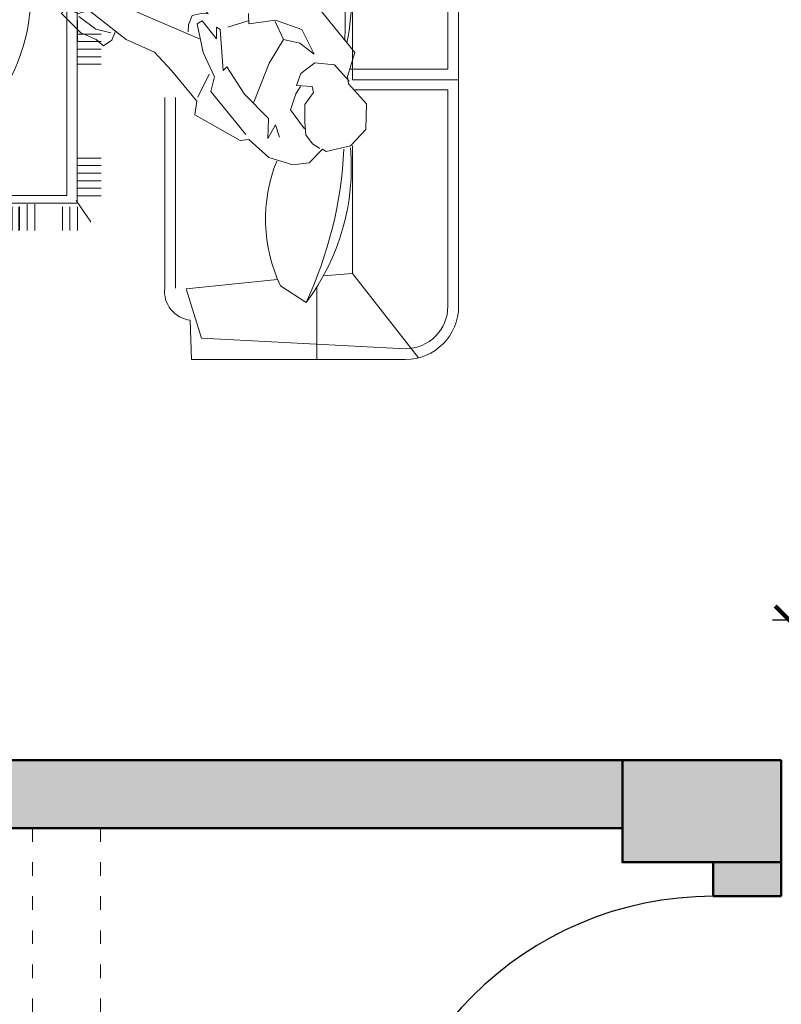
# Model space of a CAD drawing. Units: inches. Extents: x 375 to 1122, y 27 to 1069.
# Tile 5 of 155: x 599 to 667, y 313 to 400. Entities that reach past the tile are written whole.
import ezdxf

# ---------------------------------------------------------------- set-up
doc = ezdxf.new("R2010")
doc.units = ezdxf.units.IN
doc.linetypes.add('ACAD_ISO03W100', pattern=[30, 12, -18])
for name, color, linetype, lineweight in [('A-ANNO-DIMS', 2, 'Continuous', 18), ('A-COLS-PATT', 10, 'Continuous', 13), ('A-WALL-OVHD', 77, 'ACAD_ISO03W100', 18), ('A-WALL-PATT', 252, 'Continuous', 13), ('Columns', 10, 'Continuous', 50), ('Doors', 150, 'Continuous', 25), ('Furniture', 30, 'Continuous', 18), ('Walls', 250, 'Continuous', 50)]:
    doc.layers.add(name, color=color, linetype=linetype, lineweight=lineweight)
doc.styles.get("Standard").update_dxf_attribs({"font": 'arial.ttf'})
doc.dimstyles.new('ISO-25', dxfattribs={"dimtxt": 12, "dimasz": 2.5, "dimexe": 1.5, "dimexo": 1.5, "dimtad": 1, "dimdec": 1, "dimlunit": 3, "dimtxsty": 'Standard', "dimblk": 'ARCHTICK', "dimcen": 2.5, "dimadec": 0, "dimazin": 0, "dimtfac": 1, "dimtdec": 1, "dimtmove": 0, "dimatfit": 3, "dimfxl": 1.5, "dimfxlon": 1, "dimarcsym": 0})

# ---------------------------------------------------------------- blocks, each defined once
blk = doc.blocks.new('*U10')
for p, q in [((-30, 0), (-30, 4)), ((0, 0), (0, 4))]:
    blk.add_line(p, q)
blk.add_lwpolyline([(0, 0), (0, -30), (-1.75, -30), (-1.75, 0)], close=True)
blk.add_arc((0, 0), 30, 180, 270)
blk = doc.blocks.new('A$C4DC51D13')
for p, q in [((3265.3, 2996.2), (1188.4, 2996.2)), ((1895.2, 2134), (1895.2, 2996.2)), ((2559.6, 2996.2), (2559.6, 2617.8)), ((1188.4, 2962.7), (1862.1, 2962.7)), ((1862.1, 2134), (1862.1, 2962.7)), ((1928.3, 2961.6), (2524.2, 2961.6)), ((1928.3, 2134), (1928.3, 2961.6)), ((2524.2, 2961.6), (2524.2, 2658.6)), ((2590.4, 2962.7), (2590.4, 2654.5)), ((3265.3, 2962.7), (2590.4, 2962.7)), ((277.4, 2939.6), (277.4, 2141.8)), ((943, 2103.5), (943, 2936.7)), ((1018.2, 2892.3), (232.2, 2892.3)), ((3778.5, 2897), (3631.2, 2747.3)), ((4008.9, 2375.5), (3778.5, 2897)), ((4156.2, 2525.2), (3778.5, 2897)), ((304, 2865.7), (304, 2253.3)), ((916.4, 2865.7), (304, 2865.7)), ((916.4, 2253.3), (916.4, 2865.7)), ((1290.4, 2664.8), (1028, 2870.9)), ((3163.3, 2664.8), (3425.7, 2870.9)), ((1022.9, 2163.8), (1022.9, 2830.3)), ((1056, 2830.3), (1081, 2194.8)), ((3397.7, 2830.3), (3364.5, 2194.8)), ((3430.8, 2163.8), (3430.8, 2830.3)), ((4008.9, 2375.5), (3631.2, 2747.3)), ((423.7, 2370.8), (776.6, 2723.7)), ((427.4, 2727.4), (772.8, 2367.1)), ((502.2, 2648.3), (502.2, 2701.8)), ((506.4, 2652.2), (506.4, 2704.4)), ((510.6, 2655.8), (510.6, 2706.9)), ((514.9, 2659.2), (514.9, 2709.2)), ((519.1, 2662.3), (519.1, 2711.3)), ((523.3, 2665.1), (523.3, 2713.4)), ((527.5, 2667.8), (527.5, 2715.2)), ((531.8, 2670.2), (531.8, 2717)), ((536, 2672.5), (536, 2718.7)), ((540.2, 2674.6), (540.2, 2720.2)), ((544.4, 2676.5), (544.4, 2721.6)), ((548.7, 2678.2), (548.7, 2722.9)), ((650.1, 2678.8), (650.1, 2723.3)), ((654.3, 2677.1), (654.3, 2722)), ((658.6, 2675.2), (658.6, 2720.7)), ((662.8, 2673.2), (662.8, 2719.2)), ((667, 2671), (667, 2717.6)), ((668.5, 2670.2), (668.5, 2717)), ((671.2, 2668.6), (671.2, 2715.9)), ((672.7, 2667.8), (672.7, 2715.2)), ((675.5, 2666.1), (675.5, 2714)), ((676.9, 2665.1), (676.9, 2713.4)), ((679.7, 2663.3), (679.7, 2712)), ((681.1, 2662.3), (681.1, 2711.3)), ((683.9, 2660.3), (683.9, 2709.9)), ((685.4, 2659.2), (685.4, 2709.2)), ((688.1, 2657), (688.1, 2707.7)), ((689.6, 2655.8), (689.6, 2706.9)), ((692.4, 2653.5), (692.4, 2705.3)), ((693.8, 2652.2), (693.8, 2704.4)), ((696.6, 2649.6), (696.6, 2702.7)), ((698, 2648.3), (698, 2701.8)), ((465.8, 2671.5), (534.1, 2671.5)), ((468.4, 2596.6), (468.4, 2674.3)), ((469.8, 2675.7), (542.8, 2675.7)), ((472.6, 2606.7), (472.6, 2678.5)), ((476.8, 2615), (476.8, 2682.5)), ((481, 2622.2), (481, 2686.2)), ((485.3, 2628.5), (485.3, 2689.7)), ((489.5, 2634.2), (489.5, 2693)), ((493.7, 2639.3), (493.7, 2696.1)), ((497.9, 2644), (497.9, 2699.1)), ((657.4, 2675.7), (730.4, 2675.7)), ((734.5, 2671.5), (666.1, 2671.5)), ((666.1, 2671.5), (734.5, 2671.5)), ((700.8, 2645.5), (700.8, 2700)), ((702.3, 2644), (702.3, 2699.1)), ((705, 2641), (705, 2697.2)), ((706.5, 2639.3), (706.5, 2696.1)), ((709.3, 2636), (709.3, 2694.1)), ((710.7, 2634.2), (710.7, 2693)), ((713.5, 2630.5), (713.5, 2690.9)), ((714.9, 2628.5), (714.9, 2689.7)), ((717.7, 2624.4), (717.7, 2687.4)), ((719.2, 2622.2), (719.2, 2686.2)), ((722, 2617.6), (722, 2683.8)), ((723.4, 2615), (723.4, 2682.5)), ((726.2, 2609.7), (726.2, 2679.9)), ((727.6, 2606.7), (727.6, 2678.5)), ((730.4, 2600.3), (730.4, 2675.7)), ((731.9, 2596.6), (731.9, 2674.3)), ((734.6, 2588.4), (734.6, 2671.3)), ((3631.7, 2676.6), (3938.2, 2375)), ((443, 2453.4), (443, 2641.1)), ((443.5, 2641.9), (496, 2641.9)), ((446.1, 2646.1), (500, 2646.1)), ((447.2, 2446.7), (447.2, 2647.8)), ((448.9, 2650.4), (504.4, 2650.4)), ((451.5, 2440.6), (451.5, 2654)), ((451.9, 2654.6), (509.2, 2654.6)), ((455.1, 2658.8), (514.4, 2658.8)), ((455.7, 2434.9), (455.7, 2659.6)), ((458.4, 2663.1), (520.2, 2663.1)), ((459.9, 2558.8), (459.9, 2664.9)), ((462, 2667.3), (526.7, 2667.3)), ((464.1, 2583.3), (464.1, 2669.7)), ((489.5, 2667.3), (489.5, 2633.5)), ((738.2, 2667.3), (673.5, 2667.3)), ((673.5, 2667.3), (738.2, 2667.3)), ((741.8, 2663.1), (680, 2663.1)), ((680, 2663.1), (741.8, 2663.1)), ((745.2, 2658.8), (685.8, 2658.8)), ((685.8, 2658.8), (745.2, 2658.8)), ((748.3, 2654.6), (691, 2654.6)), ((691, 2654.6), (748.3, 2654.6)), ((751.3, 2650.4), (695.8, 2650.4)), ((695.8, 2650.4), (751.3, 2650.4)), ((754.1, 2646.1), (700.2, 2646.1)), ((700.2, 2646.1), (754.1, 2646.1)), ((756.7, 2641.9), (704.2, 2641.9)), ((704.2, 2641.9), (756.7, 2641.9)), ((736.1, 2583.3), (736.1, 2669.7)), ((738.9, 2570.4), (738.9, 2666.6)), ((740.3, 2558.8), (740.3, 2664.9)), ((743.1, 2433.1), (743.1, 2661.5)), ((744.5, 2434.9), (744.5, 2659.6)), ((747.3, 2438.6), (747.3, 2656)), ((748.8, 2440.6), (748.8, 2654)), ((751.5, 2444.5), (751.5, 2650)), ((753, 2446.7), (753, 2647.8)), ((755.8, 2451.1), (755.8, 2643.5)), ((757.2, 2453.4), (757.2, 2641.1)), ((1283.3, 2574.2), (1290.4, 2664.8)), ((1290.4, 2664.8), (1894.7, 2664.8)), ((1895.2, 2663.7), (2557.3, 2663.7)), ((2603.6, 2664.8), (2559, 2664.8)), ((3163.3, 2664.8), (2764.7, 2664.8)), ((3170.4, 2574.2), (3163.3, 2664.8)), ((429.1, 2612.3), (475.4, 2612.3)), ((430.3, 2479), (430.3, 2615.5)), ((430.7, 2616.6), (477.7, 2616.6)), ((432.5, 2620.8), (480.2, 2620.8)), ((434.5, 2469.3), (434.5, 2625.2)), ((434.5, 2625), (482.9, 2625)), ((436.5, 2629.2), (485.8, 2629.2)), ((438.7, 2633.5), (488.9, 2633.5)), ((438.8, 2460.9), (438.8, 2633.6)), ((441, 2637.7), (492.3, 2637.7)), ((759.2, 2637.7), (707.9, 2637.7)), ((707.9, 2637.7), (759.2, 2637.7)), ((761.5, 2633.5), (711.3, 2633.5)), ((711.3, 2633.5), (761.5, 2633.5)), ((763.7, 2629.2), (714.4, 2629.2)), ((714.4, 2629.2), (763.7, 2629.2)), ((765.8, 2625), (717.3, 2625)), ((767.7, 2620.8), (720, 2620.8)), ((769.5, 2616.6), (722.5, 2616.6)), ((771.1, 2612.3), (724.8, 2612.3)), ((760, 2458.3), (760, 2636.3)), ((761.4, 2460.9), (761.4, 2633.6)), ((764.2, 2466.3), (764.2, 2628.2)), ((765.7, 2469.3), (765.7, 2625.2)), ((1798, 2530.2), (1812.1, 2637.9)), ((419.8, 2578.5), (462.9, 2578.5)), ((420.6, 2582.7), (464, 2582.7)), ((421.5, 2587), (465.2, 2587)), ((422.5, 2591.2), (466.5, 2591.2)), ((423.6, 2595.4), (467.9, 2595.4)), ((424.8, 2599.7), (469.6, 2599.7)), ((426.1, 2603.9), (471.3, 2603.9)), ((426.1, 2490.7), (426.1, 2603.9)), ((427.5, 2608.1), (473.3, 2608.1)), ((772.7, 2608.1), (726.9, 2608.1)), ((774.1, 2603.9), (728.9, 2603.9)), ((775.4, 2599.7), (730.7, 2599.7)), ((776.6, 2595.4), (732.3, 2595.4)), ((777.7, 2591.2), (733.7, 2591.2)), ((778.7, 2587), (735.1, 2587)), ((779.6, 2582.7), (736.2, 2582.7)), ((780.4, 2578.5), (737.3, 2578.5)), ((1895.5, 2582.2), (1932.3, 2494.6)), ((417.1, 2548.9), (459.4, 2548.9)), ((417.2, 2553.2), (459.6, 2553.2)), ((417.4, 2557.4), (459.8, 2557.4)), ((417.7, 2561.6), (460.2, 2561.6)), ((418.1, 2565.8), (460.7, 2565.8)), ((418.5, 2570.1), (461.3, 2570.1)), ((419.1, 2574.3), (462.1, 2574.3)), ((781.1, 2574.3), (738.2, 2574.3)), ((781.7, 2570.1), (738.9, 2570.1)), ((782.2, 2565.8), (739.6, 2565.8)), ((782.5, 2561.6), (740.1, 2561.6)), ((782.8, 2557.4), (740.4, 2557.4)), ((783, 2553.2), (740.7, 2553.2)), ((783.1, 2548.9), (740.8, 2548.9)), ((1022.9, 2554.4), (1249.6, 2554.4)), ((3430.8, 2554.4), (3204.1, 2554.4)), ((417.1, 2544.7), (459.5, 2544.7)), ((417.2, 2540.5), (459.6, 2540.5)), ((417.5, 2536.3), (459.9, 2536.3)), ((417.8, 2532), (460.3, 2532)), ((418.2, 2527.8), (460.8, 2527.8)), ((418.7, 2523.6), (461.4, 2523.6)), ((419.3, 2519.4), (462.2, 2519.4)), ((459.9, 2429.7), (459.9, 2535.7)), ((781, 2519.4), (738, 2519.4)), ((781.6, 2523.6), (738.8, 2523.6)), ((782.1, 2527.8), (739.4, 2527.8)), ((782.5, 2532), (740, 2532)), ((740.3, 2429.7), (740.3, 2535.7)), ((782.8, 2536.3), (740.4, 2536.3)), ((783, 2540.5), (740.6, 2540.5)), ((783.1, 2544.7), (740.8, 2544.7)), ((1200, 2520.5), (1251.9, 2440.8)), ((2559, 2535.8), (2557.3, 2535.8)), ((3253.7, 2520.5), (3201.8, 2440.8)), ((4008.9, 2375.5), (4156.2, 2525.2)), ((1243.2, 2146.7), (1272.2, 2431.8)), ((3210.5, 2146.7), (3181.5, 2431.8)), ((304, 2253.3), (916.4, 2253.3)), ((242.9, 2226.7), (1018.2, 2226.7)), ((1081, 2194.8), (1243.2, 2146.7)), ((3364.5, 2194.8), (3210.5, 2146.7)), ((1145.1, 2159.3), (1022.9, 2163.8)), ((1145.1, 2159.3), (1243.2, 2146.7)), ((2590.4, 2164.3), (2590.4, 2134)), ((3308.6, 2159.3), (3210.5, 2146.7)), ((3308.6, 2159.3), (3430.8, 2163.8)), ((498.8, 1837.1), (382.1, 2139.5)), ((1040.3, 1942.9), (421.2, 2132.6)), ((1244.8, 2113), (1243.2, 2146.7)), ((3208.9, 2113), (3210.5, 2146.7)), ((411.8, 2101.9), (992.6, 1890.2)), ((1839.5, 2113), (1244.8, 2113)), ((2308.5, 2111.9), (1950.4, 2111.9)), ((2614.2, 2113), (3208.9, 2113)), ((1839.5, 2079.9), (1244.8, 2079.9)), ((2322.1, 2078.8), (1950.4, 2078.8)), ((2614.2, 2079.9), (3208.9, 2079.9)), ((220.3, 2026), (19.3, 1370.1)), ((677.4, 2054.1), (612.9, 1843.6)), ((251.1, 2016.6), (37.1, 1314.7)), ((1009.7, 1828.1), (1040.3, 1942.9)), ((658.5, 1880), (717.8, 1809.1)), ((992.6, 1890.2), (993.4, 1733.4)), ((1158.3, 1784.3), (1158.3, 1858.2)), ((1181.8, 1784.3), (1181.8, 1858.2)), ((1205.3, 1784.3), (1205.3, 1858.2)), ((1228.8, 1784.3), (1228.8, 1858.2)), ((1252.2, 1784.3), (1252.2, 1858.2)), ((1319.4, 1784.3), (1319.4, 1858.2)), ((1342.9, 1784.3), (1342.9, 1858.2)), ((1366.3, 1784.3), (1366.3, 1858.2)), ((1389.8, 1784.3), (1389.8, 1858.2)), ((1413.3, 1784.3), (1413.3, 1858.2)), ((1436.8, 1784.3), (1436.8, 1858.2)), ((1460.2, 1784.3), (1460.2, 1858.2)), ((1483.7, 1784.3), (1483.7, 1858.2)), ((1507.2, 1784.3), (1507.2, 1858.2)), ((1530.7, 1784.3), (1530.7, 1858.2)), ((1554.1, 1784.3), (1554.1, 1858.2)), ((1577.6, 1784.3), (1577.6, 1858.2)), ((1714.2, 1784.3), (1714.2, 1858.2)), ((1737.6, 1784.3), (1737.6, 1858.2)), ((1761.1, 1784.3), (1761.1, 1858.2)), ((1784.6, 1784.3), (1784.6, 1858.2)), ((1808.1, 1784.3), (1808.1, 1858.2)), ((1831.5, 1784.3), (1831.5, 1858.2)), ((1855, 1784.3), (1855, 1858.2)), ((1878.5, 1784.3), (1878.5, 1858.2)), ((1902, 1784.3), (1902, 1858.2)), ((2050.7, 1784.3), (2050.7, 1858.2)), ((2074.2, 1784.3), (2074.2, 1858.2)), ((2097.7, 1784.3), (2097.7, 1858.2)), ((2121.1, 1784.3), (2121.1, 1858.2)), ((2144.6, 1784.3), (2144.6, 1858.2)), ((2168.1, 1784.3), (2168.1, 1858.2)), ((2191.6, 1782.4), (2191.6, 1856.3)), ((2238.5, 1785.1), (2238.5, 1859)), ((2262, 1784.3), (2262, 1858.2)), ((2285.4, 1784.3), (2285.4, 1858.2)), ((2543.7, 1784.3), (2543.7, 1858.2)), ((2567.1, 1784.3), (2567.1, 1858.2)), ((2590.6, 1784.3), (2590.6, 1858.2)), ((2614.1, 1784.3), (2614.1, 1858.2)), ((2661, 1784.3), (2661, 1858.2)), ((2684.5, 1784.3), (2684.5, 1858.2)), ((2708, 1772.3), (2708, 1858.2)), ((2731.5, 1784.3), (2731.5, 1858.2)), ((2754.9, 1784.3), (2754.9, 1858.2)), ((2778.4, 1784.3), (2778.4, 1858.2)), ((2801.9, 1784.3), (2801.9, 1858.2)), ((2825.4, 1784.3), (2825.4, 1858.2)), ((2848.8, 1784.3), (2848.8, 1858.2)), ((2872.3, 1784.3), (2872.3, 1858.2)), ((2895.8, 1784.3), (2895.8, 1858.2)), ((2919.3, 1784.3), (2919.3, 1858.2)), ((2942.7, 1784.3), (2942.7, 1858.2)), ((2966.2, 1744.8), (2966.2, 1858.2)), ((2989.7, 1784.3), (2989.7, 1858.2)), ((3013.2, 1772.3), (3013.2, 1858.2)), ((3036.6, 1784.3), (3036.6, 1858.2)), ((3060.1, 1784.3), (3060.1, 1858.2)), ((3083.6, 1784.3), (3083.6, 1858.2)), ((498.8, 1837.1), (341.4, 1323.6)), ((584.9, 1817.9), (498.8, 1837.1)), ((1009.7, 1828.1), (993.4, 1733.4)), ((1158.3, 1821.3), (1158.5, 487.7)), ((2215, 1785.7), (2215, 1832.3)), ((993.4, 1733.4), (720.4, 1787.6)), ((1166.1, 1769.7), (1091.8, 1794.5)), ((1162.1, 1754.9), (1088.2, 1754.9)), ((3248.4, 1772.3), (1158.5, 1772.3)), ((3248.4, 487.7), (3248.4, 1772.3)), ((3248.8, 1760.8), (3322.7, 1760.8)), ((1024.2, 1722.3), (842.3, 1125.2)), ((1024.2, 1722.3), (993.4, 1733.4)), ((1162.1, 1741.1), (1088.2, 1741.1)), ((1196, 511), (1196, 1744.8)), ((1196, 1744.8), (3215.6, 1744.8)), ((3215.6, 511), (3215.6, 1744.8)), ((3248.8, 1737.3), (3322.7, 1737.3)), ((3600.6, 1621.7), (3605.1, 1743.8)), ((3605.1, 1743.8), (4271.6, 1743.8)), ((3995.7, 1743.8), (3995.7, 1517.1)), ((4106.1, 1476.4), (4312.2, 1738.8)), ((873.1, 1115.8), (1055, 1712.9)), ((1162.1, 1717.6), (1088.2, 1717.6)), ((1162.1, 1708), (1088.2, 1708)), ((3248.8, 1713.8), (3322.7, 1713.8)), ((3248.8, 1690.4), (3322.7, 1690.4)), ((4271.6, 1710.7), (3636.1, 1685.8)), ((1162.1, 1684.5), (1088.2, 1684.5)), ((3248.8, 1666.9), (3322.7, 1666.9)), ((3636.1, 1685.8), (3588, 1523.6)), ((3248.8, 1643.4), (3322.7, 1643.4)), ((3248.8, 1619.9), (3322.7, 1619.9)), ((3600.6, 1621.7), (3588, 1523.6)), ((4404, 1578.3), (4404, 904.6)), ((4437.5, 165.9), (4437.5, 1578.3)), ((1701.7, 1530), (1701.7, 911.2)), ((3248.8, 1513.8), (3322.7, 1513.8)), ((3248.8, 1513.3), (3322.7, 1513.3)), ((3521.2, 1130.7), (3521.2, 1521.9)), ((3554.3, 1131.4), (3554.3, 1521.9)), ((3588, 1523.6), (3873.1, 1494.5)), ((1162.1, 1492.9), (1088.2, 1492.9)), ((1162.1, 1483.3), (1088.2, 1483.3)), ((1737.7, 1483.1), (1737.7, 911.2)), ((2593.1, 907.9), (2593.1, 1490.3)), ((2629.1, 907.9), (2629.1, 1503.1)), ((3248.8, 1490.4), (3322.7, 1490.4)), ((3248.8, 1489.9), (3322.7, 1489.9)), ((4015.5, 1483.4), (4106.1, 1476.4)), ((4106.1, 1476.4), (4106.1, 872.1)), ((1162.1, 1459.8), (1088.2, 1459.8)), ((1162.1, 1446), (1088.2, 1446)), ((2674.6, 1449.9), (1641, 1449.9)), ((1888.1, 1449.9), (1701.7, 1263.5)), ((1856.2, 1449.9), (1701.7, 1295.4)), ((1715.1, 1449.9), (1701.7, 1436.5)), ((2343.3, 1449.9), (1855.3, 961.9)), ((2629.1, 1449), (2142, 961.9)), ((2325.1, 1449.9), (2154.2, 1279.1)), ((2461.6, 1449.9), (2177, 1165.3)), ((3248.8, 1466.9), (3322.7, 1466.9)), ((3248.8, 1443.4), (3322.7, 1443.4)), ((1162.1, 1412.8), (1088.2, 1412.8)), ((2674.6, 1413.9), (1641, 1413.9)), ((3248.8, 1419.9), (3322.7, 1419.9)), ((1162.1, 1399), (1088.2, 1399)), ((3250, 1407.8), (3519, 1407.8)), ((6.3, 1324.2), (19.3, 1370.2)), ((1162.1, 1375.5), (1088.2, 1375.5)), ((1162.1, 1352.1), (1088.2, 1352.1)), ((3248.8, 1359), (3322.7, 1359)), ((342.8, 1324.6), (76.7, 1139.6)), ((843, 1127.6), (342.8, 1324.6)), ((479.3, 1327.3), (375.2, 1344.9)), ((1162.1, 1342.9), (1088.2, 1342.9)), ((1162.1, 1342.4), (1088.2, 1342.4)), ((3248.8, 990.8), (3248.4, 1328.4)), ((1162.1, 1319.4), (1088.2, 1319.4)), ((1162.1, 1318.9), (1088.2, 1318.9)), ((1162.1, 1296), (1088.2, 1296)), ((1162.1, 1295.5), (1088.2, 1295.5)), ((3248.8, 1312.1), (3322.7, 1312.1)), ((3248.8, 1302.3), (3322.7, 1302.3)), ((3250, 1317.8), (3519, 1317.8)), ((369.2, 1044.8), (442.9, 1285.2)), ((1196, 1272.5), (1088.2, 1272.5)), ((1162.1, 1272), (1088.2, 1272)), ((2629.1, 1280.5), (2310.5, 961.9)), ((1162.1, 1249), (1088.2, 1249)), ((1162.1, 1248.5), (1088.2, 1248.5)), ((3248.8, 1249), (3322.7, 1249)), ((3248.8, 1248.5), (3322.7, 1248.5)), ((3248.8, 1239.3), (3322.7, 1239.3)), ((3248.8, 1238.8), (3322.7, 1238.8)), ((1162.1, 1225.5), (1088.2, 1225.5)), ((1162.1, 1202.1), (1088.2, 1202.1)), ((3248.8, 1225.5), (3322.7, 1225.5)), ((3248.8, 1202.1), (3322.7, 1202.1)), ((1196, 1178.6), (1088.2, 1178.6)), ((3248.8, 1178.6), (3322.7, 1178.6)), ((122.4, 1154.1), (719.7, 996.3)), ((1162.1, 1155.1), (1088.2, 1155.1)), ((1728.6, 1158.4), (1701.7, 1131.5)), ((3248.8, 1155.1), (3322.7, 1155.1)), ((732, 933.5), (112.9, 1123.3)), ((719.7, 996.3), (810.6, 1133.2)), ((771, 1045.7), (810.6, 1133.2)), ((842.3, 1125.2), (810.6, 1133.2)), ((1162.1, 1131.6), (1088.2, 1131.6)), ((1162.1, 1108.2), (1088.2, 1108.2)), ((3248.8, 1131.6), (3322.7, 1131.6)), ((3248.8, 1108.2), (3322.7, 1108.2)), ((1162.1, 1084.7), (1088.2, 1084.7)), ((771, 1045.7), (732, 933.5)), ((1196, 1061.2), (1088.2, 1061.2)), ((1926.6, 1051.5), (1837.1, 961.9)), ((1162.1, 1037.7), (1088.2, 1037.7)), ((1162.1, 1014.3), (1088.2, 1014.3)), ((1648.3, 1019.6), (2616.7, 1019.6)), ((3248.8, 1014.3), (3322.7, 1014.3)), ((2006.3, 994.6), (1973.6, 961.9)), ((2629.1, 1012), (2579, 961.9)), ((3248.8, 990.8), (3322.7, 990.8)), ((1196, 967.3), (1088.2, 967.3)), ((1648.3, 961.9), (2681.9, 961.9)), ((2459.2, 974.1), (2447, 961.9)), ((3248.8, 967.3), (3322.7, 967.3)), ((1162.1, 943.8), (1088.2, 943.8)), ((3248.8, 943.8), (3322.7, 943.8)), ((1162.1, 920.4), (1088.2, 920.4)), ((3248.8, 920.4), (3322.7, 920.4)), ((4097.4, 904.6), (4404, 904.6)), ((1196, 860.5), (1088.2, 860.5)), ((4106.1, 871.5), (4437.5, 871.5)), ((1162.1, 837), (1088.2, 837)), ((4404, 840.7), (4110.5, 840.7)), ((4404, 165.9), (4404, 840.7)), ((1162.1, 813.5), (1088.2, 813.5)), ((3521.2, 816.9), (3521.2, 222.3)), ((3554.3, 816.9), (3554.3, 222.3)), ((1162.1, 790), (1031.8, 790)), ((1196, 766.6), (1088.2, 766.6)), ((1162.1, 743.1), (1088.2, 743.1)), ((1162.1, 719.6), (1088.2, 719.6)), ((4106.1, 267.8), (4106.1, 666.5)), ((1162.1, 627.8), (1088.2, 627.8)), ((3248.8, 627.8), (3322.7, 627.8)), ((1162.1, 604.4), (1088.2, 604.4)), ((3248.8, 604.4), (3322.7, 604.4)), ((1162.1, 580.9), (1034.2, 580.9)), ((1162.1, 557.4), (1088.2, 557.4)), ((3248.8, 580.9), (3322.7, 580.9)), ((3248.8, 557.4), (3322.7, 557.4)), ((1162.1, 533.9), (1088.2, 533.9)), ((3248.8, 533.9), (3322.7, 533.9)), ((1162.1, 510.5), (1088.2, 510.5)), ((1162, 495.1), (1116.6, 429)), ((3215.6, 511), (1196, 511)), ((1334.6, 511), (1334.6, 402.4)), ((1381.6, 511), (1381.6, 402.4)), ((2059.5, 511), (2059.5, 402.4)), ((2106.4, 511), (2106.4, 402.4)), ((2669.8, 511), (2669.8, 402.4)), ((3244.9, 495.1), (3290.3, 429)), ((3248.8, 510.5), (3322.7, 510.5)), ((1158.5, 487.7), (3248.4, 487.7)), ((1167.1, 476.3), (1167.1, 402.4)), ((1190.6, 476.3), (1190.6, 402.4)), ((1214, 476.3), (1214, 402.4)), ((1237.5, 476.3), (1237.5, 402.4)), ((1311.1, 487.7), (1311.1, 402.4)), ((1358.1, 476.3), (1358.1, 402.4)), ((1405, 476.3), (1405, 402.4)), ((1428.5, 487.7), (1428.5, 402.4)), ((1452, 476.3), (1452, 402.4)), ((1475.5, 476.3), (1475.5, 402.4)), ((1498.9, 487.7), (1498.9, 402.4)), ((1522.4, 487.7), (1522.4, 402.4)), ((1545.9, 476.3), (1545.9, 402.4)), ((1569.4, 476.3), (1569.4, 402.4)), ((1592.8, 476.3), (1592.8, 402.4)), ((1616.3, 476.3), (1616.3, 402.4)), ((1639.8, 476.3), (1639.8, 402.4)), ((1663.3, 487.7), (1663.3, 402.4)), ((1757.8, 487.7), (1757.8, 402.4)), ((1781.3, 487.7), (1781.3, 402.4)), ((1804.8, 476.3), (1804.8, 402.4)), ((1828.2, 476.3), (1828.2, 402.4)), ((1851.7, 476.3), (1851.7, 402.4)), ((1875.2, 476.3), (1875.2, 402.4)), ((1898.7, 476.3), (1898.7, 402.4)), ((1922.1, 487.7), (1922.1, 402.4)), ((2036, 487.7), (2036, 402.4)), ((2082.9, 476.3), (2082.9, 402.4)), ((2129.9, 476.3), (2129.9, 402.4)), ((2153.4, 487.7), (2153.4, 402.4)), ((2176.8, 476.3), (2176.8, 402.4)), ((2200.3, 476.3), (2200.3, 402.4)), ((2223.8, 487.7), (2223.8, 402.4)), ((2247.2, 487.7), (2247.2, 402.4)), ((2270.7, 476.3), (2270.7, 402.4)), ((2294.2, 476.3), (2294.2, 402.4)), ((2317.7, 476.3), (2317.7, 402.4)), ((2341.1, 476.3), (2341.1, 402.4)), ((2364.6, 476.3), (2364.6, 402.4)), ((2388.1, 487.7), (2388.1, 402.4)), ((2411.6, 476.3), (2411.6, 402.4)), ((2435, 476.3), (2435, 402.4)), ((2458.5, 476.3), (2458.5, 402.4)), ((2482, 487.7), (2482, 402.4)), ((2505.5, 487.7), (2505.5, 402.4)), ((2528.9, 476.3), (2528.9, 402.4)), ((2552.4, 476.3), (2552.4, 402.4)), ((2575.9, 476.3), (2575.9, 402.4)), ((2599.4, 476.3), (2599.4, 402.4)), ((2622.8, 476.3), (2622.8, 402.4)), ((2646.3, 476.3), (2646.3, 402.4)), ((2693.3, 476.3), (2693.3, 402.4)), ((2716.7, 476.3), (2716.7, 402.4)), ((2738, 476.3), (2738, 402.4)), ((2740.2, 487.7), (2740.2, 402.4)), ((2761.5, 476.3), (2761.5, 402.4)), ((2763.7, 476.3), (2763.7, 402.4)), ((2784.9, 487.7), (2784.9, 402.4)), ((2787.2, 476.3), (2787.2, 402.4)), ((2808.4, 476.3), (2808.4, 402.4)), ((2810.6, 476.3), (2810.6, 402.4)), ((2831.9, 476.3), (2831.9, 402.4)), ((2834.1, 476.3), (2834.1, 402.4)), ((2855.4, 476.3), (2855.4, 402.4)), ((2857.6, 476.3), (2857.6, 402.4)), ((2878.8, 476.3), (2878.8, 402.4)), ((2881.1, 476.3), (2881.1, 402.4)), ((2902.3, 476.3), (2902.3, 402.4)), ((2904.5, 487.7), (2904.5, 402.4)), ((2925.8, 476.3), (2925.8, 402.4)), ((2928, 476.3), (2928, 402.4)), ((2949.3, 476.3), (2949.3, 402.4)), ((2951.5, 476.3), (2951.5, 402.4)), ((2972.7, 476.3), (2972.7, 402.4)), ((2975, 476.3), (2975, 402.4)), ((2996.2, 476.3), (2996.2, 402.4)), ((2998.4, 476.3), (2998.4, 402.4)), ((3019.7, 476.3), (3019.7, 402.4)), ((3021.9, 487.7), (3021.9, 402.4)), ((3043.2, 476.3), (3043.2, 402.4)), ((3045.4, 476.3), (3045.4, 402.4)), ((3066.6, 476.3), (3066.6, 402.4)), ((3068.9, 476.3), (3068.9, 402.4)), ((3092.3, 476.3), (3092.3, 402.4)), ((3092.7, 484.5), (3092.7, 410.6)), ((3115.8, 476.3), (3115.8, 402.4)), ((3116.2, 484.5), (3116.2, 410.6)), ((3202.2, 476.3), (3202.2, 402.4)), ((3225.7, 476.3), (3225.7, 402.4)), ((3249.2, 476.3), (3249.2, 402.4)), ((3588, 220.6), (3873.1, 249.7)), ((4015.5, 260.8), (4106.1, 267.8)), ((4106.1, 267.8), (4312.2, 5.4)), ((3636.1, 66.6), (3588, 220.6)), ((3961.8, 177.4), (3882.1, 229.3)), ((3995.7, 0.4), (3995.7, 227)), ((3600.6, 122.5), (3605.1, 0.4)), ((4271.6, 33.5), (3636.1, 66.6)), ((3605.1, 0.4), (4271.6, 0.4))]:
    blk.add_line(p, q)
at = {"linetype": 'ByBlock'}
for points in [[(2342.9, 1843.9), (2352.5, 1810.4), (2340.1, 1777.7), (2351.8, 1757), (2412.3, 1818), (2433.1, 1866.4), (2453.1, 1889.5), (2436, 1914.7), (2407.6, 1926.2), (2433.7, 1959.9), (2473.1, 2048.3), (2530.6, 2101.1), (2625.9, 2180.3), (2669, 2174.2), (2748.1, 2315.4), (2745.8, 2342.6), (2801.2, 2404.9), (2823.9, 2479.6), (2818.4, 2529.9), (2775.1, 2571.7), (2782.4, 2583.3), (2765.2, 2658.8), (2714.5, 2706.9), (2634.6, 2708.6), (2571.9, 2652.6), (2548.8, 2649.4), (2474, 2672.1), (2312.9, 2542.1), (2312.9, 2341.6), (2333.9, 2336.4), (2302, 2223.9), (2313.6, 2216.6), (2297.4, 2095.7), (2309.3, 2034.9), (2320.2, 1952), (2319.3, 1929.9), (2280.8, 1863.6), (2257.7, 1842.4), (2239.2, 1825.7), (2220.1, 1798.2), (2221.6, 1713.1), (2254.3, 1700.7), (2275.9, 1729.8), (2288.6, 1768), (2313.7, 1797.6)], [(3285.2, 1088.3), (3251.7, 1078.6), (3219, 1091.1), (3198.3, 1079.4), (3259.3, 1018.8), (3307.7, 998), (3330.8, 978), (3356, 995.1), (3367.5, 1023.6), (3401.2, 997.5), (3489.6, 958), (3542.4, 900.5), (3621.6, 805.3), (3615.5, 762.2), (3756.7, 683), (3783.9, 685.3), (3846.2, 629.9), (3920.9, 607.2), (3971.2, 612.7), (4013, 656), (4024.6, 648.7), (4100.1, 665.9), (4148.2, 716.6), (4149.9, 796.5), (4093.9, 859.3), (4090.7, 882.4), (4113.4, 957.1), (3983.4, 1118.2), (3782.9, 1118.2), (3777.7, 1097.2), (3665.2, 1129.2), (3657.9, 1117.6), (3537, 1133.7), (3476.2, 1121.9), (3393.3, 1110.9), (3371.2, 1111.9), (3304.9, 1150.4), (3283.7, 1173.4), (3267, 1191.9), (3239.5, 1211), (3154.4, 1209.5), (3142, 1176.8), (3171.1, 1155.3), (3209.3, 1142.5), (3238.9, 1117.5)]]:
    blk.add_lwpolyline(points, close=True, dxfattribs=at)
for points in [[(2563.4, 2654.7), (2512.2, 2609.3), (2506.2, 2548.3), (2540.1, 2504.4), (2576.9, 2490.9), (2579.8, 2539.3), (2598.7, 2543.6), (2636.7, 2516.4), (2690.3, 2516.7), (2731.2, 2520.1), (2758.5, 2540.1), (2773, 2563.3)], [(2629.1, 2357.8), (2507, 2405.5), (2433.2, 2450.3), (2445.5, 2500.8), (2478.9, 2546.1), (2402.4, 2506.9), (2373.4, 2424.8), (2384.4, 2341.9), (2352.8, 2340.7)], [(2712.3, 2515.8), (2652.7, 2472.4), (2603.2, 2489), (2580, 2503.6)], [(2738, 2438.2), (2699.2, 2425.4), (2742.4, 2401.4), (2680.4, 2403.2), (2604.1, 2328.3), (2519.2, 2273.3), (2529.8, 2261.8), (2402.7, 2252.7), (2395.4, 2241.1), (2431.1, 2241.3), (2375.7, 2196.9), (2385.2, 2181.2), (2474.4, 2199.5), (2549.9, 2234.6), (2596.2, 2223.2), (2730.1, 2333.1)], [(2433.2, 2450.3), (2377.6, 2423.8)], [(2374.9, 2339.8), (2395.2, 2276.9)], [(2409.5, 2153), (2387.5, 2153.9), (2359, 2165.4), (2352.6, 2193.7), (2353.5, 2215.7), (2330.5, 2194.6), (2322.1, 2196.7), (2341.8, 2240.9), (2345.5, 2329.1)], [(2613.2, 2183.4), (2541.6, 2218.8)], [(2431.4, 2187.8), (2379.5, 2066.7), (2320.2, 1929.7)], [(2407.6, 1926.2), (2342.9, 1843.9)], [(2412.9, 1911.5), (2401.6, 1865.2), (2361.9, 1812.5)], [(2279.2, 1765.9), (2259.2, 1757.4), (2247.6, 1764.7), (2246.4, 1796.2), (2253.5, 1843.5)], [(3207.2, 1152), (3198.7, 1171.9), (3206, 1183.5), (3237.5, 1184.7), (3284.8, 1177.6)], [(3629.1, 999.7), (3508, 1051.6), (3371, 1110.9)], [(3594.3, 1021.6), (3595.2, 1043.7), (3606.7, 1072.1), (3635, 1078.6), (3657, 1077.6), (3635.9, 1100.6), (3638, 1109.1), (3682.2, 1089.3), (3770.4, 1085.6)], [(3367.5, 1023.6), (3285.2, 1088.3)], [(3799.1, 802), (3846.8, 924.2), (3891.6, 998), (3942.1, 985.6), (3987.4, 952.2), (3948.2, 1028.7), (3866.1, 1057.7), (3783.2, 1046.8), (3782, 1078.3)], [(3352.8, 1018.2), (3306.5, 1029.5), (3253.8, 1069.2)], [(3879.5, 693.2), (3866.7, 732), (3842.7, 688.8), (3844.5, 750.8), (3769.6, 827.1), (3714.6, 911.9), (3703.1, 901.3), (3694, 1028.4), (3682.4, 1035.7), (3682.6, 1000), (3638.2, 1055.5), (3622.5, 1045.9), (3640.8, 956.7), (3675.9, 881.2), (3664.5, 834.9), (3774.4, 701)], [(3781.1, 1056.2), (3718.2, 1035.9)], [(3891.6, 998), (3865.1, 1053.5)], [(4096, 867.7), (4050.6, 918.9), (3989.6, 924.9), (3945.7, 891.1), (3932.2, 854.2), (3980.6, 851.3), (3984.9, 832.4), (3957.7, 794.4), (3958, 740.9), (3961.4, 699.9), (3981.4, 672.7), (4004.6, 658.1)], [(3624.7, 817.9), (3660.1, 889.6)], [(3957.1, 718.8), (3913.7, 778.5), (3930.3, 827.9), (3944.9, 851.1)]]:
    blk.add_lwpolyline(points, dxfattribs=at)
for centre, radius in [((600.1, 2547.3), 183), ((600.1, 2547.3), 140.7), ((1803.2, 1372.6), 25.7), ((2527.6, 1372.6), 25.7), ((1803.2, 1039.3), 25.7), ((2527.6, 1039.3), 25.7), ((2817.9, 923.4), 31.7), ((2095.7, 858), 41)]:
    blk.add_circle(centre, radius)
for centre, radius, start, end in [((1188.4, 2830.3), 165.9, 90, 180), ((3265.3, 2830.3), 165.9, 0, 90), ((1188.4, 2830.3), 132.4, 90, 180), ((3265.3, 2830.3), 132.4, 0, 90), ((3666.8, 2712.2), 50, 135.4503, 225.4503), ((1626.8, 1949.8), 712.7, 74.928, 126.7929), ((1707.9, 1527), 1115.8, 84.6406, 117.0804), ((2192.2, 2032.6), 624.6, 69.4145, 118.3621), ((2633.9, 373.6), 2292.5, 91.8726, 91.9144), ((2832.8, 1963.1), 698.5, 52.9389, 95.0789), ((2210.2, 1780.8), 852.5, 76.866, 111.6839), ((2713.3, 1357.7), 1282.3, 65.0725, 87.2152), ((1459.9, 2882.7), 488.4, 244.7866, 313.8058), ((2216, 2892.1), 488.4, 234.4888, 282.1285), ((2993.8, 2882.7), 488.4, 248.2152, 295.2134), ((3973.2, 2410.6), 50, 225.4503, 315.4503), ((1234.5, 2169.3), 90, 186.4251, 276.5821), ((3219.2, 2169.3), 90, 263.4179, 353.5749), ((374.1, 1978.9), 160.8, 72.9571, 162.9571), ((1839.5, 2135.1), 22.1, 270, 0), ((1839.5, 2135.1), 55.2, 270, 0), ((1950.4, 2134), 55.2, 180, 270), ((1950.4, 2134), 22.1, 180, 270), ((2619.6, 2148.3), 68.5, 191.0595, 265.4426), ((2614.2, 2135.1), 22.1, 180, 270), ((374.1, 1978.9), 128.6, 72.9571, 162.9571), ((1584.7, 1047), 1245.7, 138.0296, 166.1636), ((1067.1, 1321), 692.3, 126.1642, 178.0291), ((974.8, 1747.9), 87.4, 336.375, 66.532), ((248.2, 1741.7), 474.4, 299.1514, 8.1705), ((4271.6, 1578.3), 165.9, 0, 90), ((4271.6, 1578.3), 132.4, 0, 90), ((944.2, 1233.8), 467.1, 309.4804, 56.621), ((3610.6, 1532.2), 90, 96.4251, 186.5821), ((3383, 1136.2), 721.4, 348.1046, 36.6442), ((2968.3, 1058.8), 1115.8, 356.7543, 27.0804), ((4324, 1306.8), 488.4, 154.7866, 202.7137), ((160.1, 1277), 160.8, 162.9571, 252.9571), ((160.1, 1277), 128.6, 162.9571, 252.9571), ((2517.5, 1143.6), 586.7, 287.3395, 13.1463), ((787.1, 1131.7), 87.4, 259.3822, 349.5393), ((2356.9, 1798.1), 1287.8, 212.1153, 261.9323), ((-29968.2, -49615.7), 59944, 56.743614, 57.623407), ((3404.4, 598.4), 698.5, 322.9389, 5.0789), ((2799, 717.9), 1282.3, 335.0725, 357.2152), ((4324, 437.4), 488.4, 158.2152, 205.2134), ((2591.9, -2109.1), 2694.5, 80.9842, 100.0261), ((3610.6, 212), 90, 173.4179, 263.5749), ((4271.6, 165.9), 132.4, 270, 0), ((4271.6, 165.9), 165.9, 270, 0)]:
    blk.add_arc(centre, radius, start, end)
blk = doc.blocks.new('COLUMN-14X9IN')
blk.add_lwpolyline([(0, 0), (14, 0), (14, 9), (0, 9)], close=True)
blk = doc.blocks.new('_ArchTick')
at = {"color": 0, "linetype": 'ByBlock', "const_width": 0.15}
blk.add_lwpolyline([(-0.5, -0.5), (0.5, 0.5)], dxfattribs=at)
blk = doc.blocks.new('*D59')
at = {"layer": 'A-ANNO-DIMS', "color": 0, "lineweight": -2, "transparency": 16777216}
for p, q in [((668.717, 346.851), (665.717, 346.851)), ((667.217, 346.851), (667.217, 232.348)), ((668.717, 232.348), (665.717, 232.348)), ((667.217, 232.348), (667.217, 27.496))]:
    blk.add_line(p, q, dxfattribs=at)
at = {"layer": 'Defpoints', "color": 0, "transparency": 16777216}
for p in [(684.392, 346.851), (667.217, 232.348), (684.392, 232.348)]:
    blk.add_point(p, dxfattribs=at)
at = {"layer": 'A-ANNO-DIMS', "color": 0, "lineweight": -2, "transparency": 16777216, "xscale": 2.5, "yscale": 2.5, "zscale": 2.5}
for p, rotation in [((667.217, 346.851), 90), ((667.217, 232.348), 270)]:
    blk.add_blockref('_ArchTick', p, dxfattribs=dict(at, rotation=rotation))
at = {"layer": 'A-ANNO-DIMS', "color": 0, "transparency": 16777216, "insert": (660.387, 128.672), "char_height": 12, "attachment_point": 5, "rotation": 90}
blk.add_mtext('DINING SET 9\'-6 1/2" TYP.', dxfattribs=at)
blk = doc.blocks.new('*D82')
at = {"layer": 'A-ANNO-DIMS', "color": 0, "lineweight": -2, "transparency": 16777216}
for p, q in [((401.507, 1009.528), (398.507, 1009.528)), ((400.007, 160.528), (400.007, 1009.528)), ((401.507, 160.528), (398.507, 160.528))]:
    blk.add_line(p, q, dxfattribs=at)
at = {"layer": 'Defpoints', "color": 0, "transparency": 16777216}
for p in [(400.007, 1009.528), (630.534, 1009.528), (630.534, 160.528)]:
    blk.add_point(p, dxfattribs=at)
at = {"layer": 'A-ANNO-DIMS', "color": 0, "lineweight": -2, "transparency": 16777216, "xscale": 2.5, "yscale": 2.5, "zscale": 2.5}
for p, rotation in [((400.007, 1009.528), 90), ((400.007, 160.528), 270)]:
    blk.add_blockref('_ArchTick', p, dxfattribs=dict(at, rotation=rotation))
at = {"layer": 'A-ANNO-DIMS', "color": 0, "transparency": 16777216, "insert": (393.255, 585.028), "char_height": 12, "attachment_point": 5, "rotation": 90}
blk.add_mtext('70\'-9"', dxfattribs=at)

msp = doc.modelspace()

# ---------------------------------------------------------------- hatches: boundary and pattern name
at = {"layer": 'A-COLS-PATT'}
h = msp.add_hatch(color=256, dxfattribs=at)
h.dxf.hatch_style = 1
h.paths.add_polyline_path([(512.507, 982.528), (498.507, 982.528), (498.507, 973.528), (512.507, 973.528)])
h.paths.add_polyline_path([(666.507, 982.528), (652.507, 982.528), (652.507, 973.528), (666.507, 973.528)])
h.paths.add_polyline_path([(802.007, 982.528), (788.007, 982.528), (788.007, 973.528), (802.007, 973.528)])
h.paths.add_polyline_path([(932.007, 982.528), (918.007, 982.528), (918.007, 973.528), (932.007, 973.528)])
h.paths.add_polyline_path([(507.507, 841.528), (498.507, 841.528), (498.507, 827.528), (507.507, 827.528)])
h.paths.add_polyline_path([(666.507, 844.528), (652.507, 844.528), (652.507, 835.528), (666.507, 835.528)])
h.paths.add_polyline_path([(802.007, 814.528), (788.007, 814.528), (788.007, 805.528), (802.007, 805.528)])
h.paths.add_polyline_path([(932.007, 814.528), (918.007, 814.528), (918.007, 805.528), (932.007, 805.528)])
h.paths.add_polyline_path([(507.507, 719.528), (498.507, 719.528), (498.507, 705.528), (507.507, 705.528)])
h.paths.add_polyline_path([(731.007, 676.528), (722.007, 676.528), (722.007, 662.528), (731.007, 662.528)])
h.paths.add_polyline_path([(802.007, 676.528), (788.007, 676.528), (788.007, 667.528), (802.007, 667.528)])
h.paths.add_polyline_path([(932.007, 676.528), (918.007, 676.528), (918.007, 667.528), (932.007, 667.528)])
h.paths.add_polyline_path([(932.007, 583.528), (918.007, 583.528), (918.007, 574.528), (932.007, 574.528)])
h.paths.add_polyline_path([(868.007, 583.528), (854.007, 583.528), (854.007, 574.528), (868.007, 574.528)])
h.paths.add_polyline_path([(868.007, 502.528), (854.007, 502.528), (854.007, 493.528), (868.007, 493.528)])
h.paths.add_polyline_path([(932.007, 502.528), (918.007, 502.528), (918.007, 493.528), (932.007, 493.528)])
h.paths.add_polyline_path([(672.507, 592.028), (663.507, 592.028), (663.507, 578.028), (672.507, 578.028)])
h.paths.add_polyline_path([(512.507, 589.528), (498.507, 589.528), (498.507, 580.528), (512.507, 580.528)])
h.paths.add_polyline_path([(507.507, 464.528), (498.507, 464.528), (498.507, 450.528), (507.507, 450.528)])
h.paths.add_polyline_path([(731.007, 507.528), (722.007, 507.528), (722.007, 493.528), (731.007, 493.528)])
h.paths.add_polyline_path([(802.007, 502.528), (788.007, 502.528), (788.007, 493.528), (802.007, 493.528)])
h.paths.add_polyline_path([(507.507, 342.528), (498.507, 342.528), (498.507, 328.528), (507.507, 328.528)])
h.paths.add_polyline_path([(512.507, 196.528), (498.507, 196.528), (498.507, 187.528), (512.507, 187.528)])
h.paths.add_polyline_path([(666.507, 334.528), (652.507, 334.528), (652.507, 325.528), (666.507, 325.528)])
h.paths.add_polyline_path([(666.507, 196.528), (652.507, 196.528), (652.507, 187.528), (666.507, 187.528)])
h.paths.add_polyline_path([(805.007, 196.528), (791.007, 196.528), (791.007, 187.528), (805.007, 187.528)])
h.paths.add_polyline_path([(932.007, 196.528), (918.007, 196.528), (918.007, 187.528), (932.007, 187.528)])
h.paths.add_polyline_path([(932.007, 334.528), (918.007, 334.528), (918.007, 325.528), (932.007, 325.528)])
h.paths.add_polyline_path([(805.007, 334.528), (791.007, 334.528), (791.007, 325.528), (805.007, 325.528)])
at = {"layer": 'A-WALL-PATT'}
h = msp.add_hatch(color=256, dxfattribs=at)
h.dxf.hatch_style = 1
h.paths.add_polyline_path([(962.007, 388.528), (989.007, 388.528), (989.007, 394.528), (962.007, 394.528), (932.007, 394.528), (932.007, 397.528), (923.007, 397.528), (923.007, 394.528), (842.007, 394.528), (842.007, 334.528), (839.507, 334.528), (839.507, 328.528), (854.007, 328.528), (854.007, 334.528), (848.007, 334.528), (848.007, 388.528), (953.007, 388.528), (953.007, 356.081), (962.007, 356.081), (962.007, 358.554), (989.007, 358.554), (989.007, 364.554), (962.007, 364.554)])
h.paths.add_polyline_path([(989.007, 502.528), (932.007, 502.528), (932.007, 583.528), (932.007, 593.528), (923.007, 593.528), (923.007, 583.528), (854.007, 583.528), (854.007, 556.528), (863.007, 556.528), (863.007, 574.528), (923.007, 574.528), (923.007, 502.528), (863.007, 502.528), (863.007, 520.528), (854.007, 520.528), (854.007, 502.528), (773.007, 502.528), (773.007, 493.528), (788.007, 493.528), (788.007, 402.028), (722.007, 402.028), (722.007, 373.528), (728.007, 373.528), (728.007, 396.028), (788.007, 396.028), (788.007, 373.528), (794.007, 373.528), (794.007, 430.528), (814.007, 430.528), (814.007, 436.528), (794.007, 436.528), (794.007, 493.528), (923.007, 493.528), (923.007, 487.528), (932.007, 487.528), (932.007, 493.528), (983.007, 493.528), (983.007, 473.528), (989.007, 473.528)])
h.paths.add_polyline_path([(797.007, 325.528), (805.007, 325.528), (805.007, 328.528), (807.507, 328.528), (807.507, 334.528), (791.007, 334.528), (791.007, 226.528), (770.757, 226.528), (770.757, 217.528), (791.007, 217.528), (791.007, 187.528), (855.007, 187.528), (855.007, 196.528), (797.007, 196.528)])
h.paths.add_polyline_path([(989.007, 238.528), (962.007, 238.528), (962.007, 256.424), (953.007, 256.424), (953.007, 229.528), (980.007, 229.528), (980.007, 196.528), (915.007, 196.528), (915.007, 187.528), (989.007, 187.528)])
h.paths.add_polyline_path([(962.007, 334.528), (884.007, 334.528), (884.007, 328.528), (918.007, 328.528), (918.007, 325.528), (932.007, 325.528), (932.007, 328.528), (953.007, 328.528), (953.007, 304.424), (962.007, 304.424)])
h.paths.add_polyline_path([(606.507, 283.528), (609.507, 283.528), (609.507, 289.528), (600.507, 289.528), (600.507, 196.528), (578.507, 196.528), (578.507, 187.528), (606.507, 187.528), (606.507, 196.528)])
h.paths.add_polyline_path([(666.507, 292.528), (660.507, 292.528), (660.507, 289.528), (633.507, 289.528), (633.507, 283.528), (660.507, 283.528), (660.507, 196.528), (628.007, 196.528), (628.007, 187.528), (630.534, 187.528), (630.534, 160.528), (636.534, 160.528), (636.534, 187.528), (660.507, 187.528), (660.507, 160.528), (666.507, 160.528), (666.507, 217.528), (686.757, 217.528), (686.757, 226.528), (666.507, 226.528)])
h.paths.add_polyline_path([(480.507, 256.424), (471.507, 256.424), (471.507, 238.528), (444.507, 238.528), (444.507, 187.528), (518.507, 187.528), (518.507, 196.528), (453.507, 196.528), (453.507, 229.528), (480.507, 229.528)])
h.paths.add_polyline_path([(480.507, 328.528), (652.507, 328.528), (652.507, 325.528), (660.507, 325.528), (660.507, 322.528), (666.507, 322.528), (666.507, 334.528), (507.507, 334.528), (507.507, 360.528), (498.507, 360.528), (498.507, 334.528), (471.507, 334.528), (471.507, 304.424), (480.507, 304.424)])
h.paths.add_polyline_path([(507.507, 484.528), (498.507, 484.528), (498.507, 444.528), (507.507, 444.528), (507.507, 454.528), (621.507, 454.528), (621.507, 460.528), (507.507, 460.528)])
h.paths.add_polyline_path([(672.507, 604.528), (683.257, 604.528), (683.257, 613.528), (669.507, 613.528), (669.507, 649.528), (663.507, 649.528), (663.507, 589.528), (507.507, 589.528), (507.507, 613.528), (498.507, 613.528), (498.507, 556.528), (507.507, 556.528), (507.507, 580.528), (663.507, 580.528), (663.507, 520.528), (669.507, 520.528), (669.507, 556.528), (683.257, 556.528), (683.257, 565.528), (672.507, 565.528)])
h.paths.add_polyline_path([(731.007, 667.528), (734.007, 667.528), (734.007, 676.528), (728.007, 676.528), (728.007, 715.528), (657.507, 715.528), (657.507, 709.528), (663.507, 709.528), (663.507, 673.528), (669.507, 673.528), (669.507, 709.528), (722.007, 709.528), (722.007, 613.528), (704.757, 613.528), (704.757, 604.528), (722.007, 604.528), (722.007, 565.528), (704.757, 565.528), (704.757, 556.528), (722.007, 556.528), (722.007, 502.528), (722.007, 460.528), (669.507, 460.528), (669.507, 496.528), (663.507, 496.528), (663.507, 460.528), (657.507, 460.528), (657.507, 454.528), (728.007, 454.528), (728.007, 493.528), (734.007, 493.528), (734.007, 502.528), (731.007, 502.528)])
h.paths.add_polyline_path([(986.007, 718.528), (959.007, 718.528), (959.007, 727.528), (950.007, 727.528), (950.007, 709.528), (977.007, 709.528), (977.007, 676.528), (794.007, 676.528), (794.007, 805.528), (802.007, 805.528), (802.007, 808.528), (804.507, 808.528), (804.507, 814.528), (788.007, 814.528), (788.007, 774.028), (728.007, 774.028), (728.007, 796.528), (722.007, 796.528), (722.007, 768.028), (788.007, 768.028), (788.007, 676.528), (773.007, 676.528), (773.007, 667.528), (923.007, 667.528), (923.007, 657.528), (932.007, 657.528), (932.007, 667.528), (986.007, 667.528)])
h.paths.add_polyline_path([(621.507, 715.528), (507.507, 715.528), (507.507, 733.528), (498.507, 733.528), (498.507, 715.528), (498.507, 685.528), (507.507, 685.528), (507.507, 709.528), (621.507, 709.528)])
h.paths.add_polyline_path([(666.507, 847.028), (660.507, 847.028), (660.507, 844.528), (652.507, 844.528), (652.507, 841.528), (480.507, 841.528), (480.507, 859.528), (471.507, 859.528), (471.507, 835.528), (498.507, 835.528), (498.507, 817.528), (507.507, 817.528), (507.507, 835.528), (666.507, 835.528)])
h.paths.add_polyline_path([(480.507, 940.528), (453.507, 940.528), (453.507, 973.528), (518.507, 973.528), (518.507, 982.528), (444.507, 982.528), (444.507, 931.528), (471.507, 931.528), (471.507, 907.528), (480.507, 907.528)])
h.paths.add_polyline_path([(606.507, 982.528), (578.507, 982.528), (578.507, 973.528), (600.507, 973.528), (600.507, 880.528), (609.507, 880.528), (609.507, 886.528), (606.507, 886.528)])
h.paths.add_polyline_path([(666.507, 943.528), (686.757, 943.528), (686.757, 952.528), (666.507, 952.528), (666.507, 1009.528), (660.507, 1009.528), (660.507, 982.528), (636.534, 982.528), (636.534, 1009.528), (630.534, 1009.528), (630.534, 982.528), (628.007, 982.528), (628.007, 973.528), (660.507, 973.528), (660.507, 886.528), (633.507, 886.528), (633.507, 880.528), (660.507, 880.528), (660.507, 877.028), (666.507, 877.028)])
h.paths.add_polyline_path([(986.007, 874.528), (932.007, 874.528), (932.007, 877.528), (923.007, 877.528), (923.007, 874.528), (788.007, 874.528), (788.007, 868.528), (788.007, 844.528), (794.007, 844.528), (794.007, 868.528), (839.007, 868.528), (839.007, 814.528), (836.507, 814.528), (836.507, 808.528), (851.007, 808.528), (851.007, 814.528), (845.007, 814.528), (845.007, 868.528), (986.007, 868.528)])
h.paths.add_polyline_path([(959.007, 838.554), (986.007, 838.554), (986.007, 844.554), (959.007, 844.554), (959.007, 847.028), (950.007, 847.028), (950.007, 814.528), (881.007, 814.528), (881.007, 808.528), (918.007, 808.528), (918.007, 805.528), (932.007, 805.528), (932.007, 808.528), (950.007, 808.528), (950.007, 793.528), (959.007, 793.528)])
h.paths.add_polyline_path([(986.007, 982.528), (899.007, 982.528), (899.007, 973.528), (923.007, 973.528), (923.007, 967.528), (932.007, 967.528), (932.007, 973.528), (980.007, 973.528), (980.007, 953.528), (986.007, 953.528)])
h.paths.add_polyline_path([(851.007, 982.528), (788.007, 982.528), (788.007, 952.528), (770.757, 952.528), (770.757, 943.528), (788.007, 943.528), (788.007, 910.528), (814.007, 910.528), (814.007, 916.528), (794.007, 916.528), (794.007, 973.528), (851.007, 973.528)])

# ---------------------------------------------------------------- linework, layer by layer
at = {"layer": 'A-WALL-OVHD', "ltscale": 0.1}
for p, q in [((600.507, 328.528), (600.507, 289.528)), ((606.507, 328.528), (606.507, 289.528))]:
    msp.add_line(p, q, dxfattribs=at)
at = {"layer": 'Walls'}
for p, q in [((507.507, 334.528), (666.507, 334.528)), ((666.507, 334.528), (666.507, 322.528)), ((480.507, 328.528), (652.507, 328.528)), ((652.507, 328.528), (652.507, 325.528)), ((652.507, 325.528), (660.507, 325.528)), ((660.507, 325.528), (660.507, 322.528)), ((660.507, 322.528), (666.507, 322.528))]:
    msp.add_line(p, q, dxfattribs=at)

# ---------------------------------------------------------------- block references
at = {"layer": 'Columns', "rotation": 180}
msp.add_blockref('COLUMN-14X9IN', (666.508, 334.527), dxfattribs=at)
at = {"layer": 'Doors', "rotation": 270}
msp.add_blockref('*U10', (660.507, 292.528), dxfattribs=at)
at = {"layer": 'Furniture', "xscale": 0.0282665567793757, "yscale": 0.0282665567793757, "zscale": 0.0282665567793757}
msp.add_blockref('A$C4DC51D13', (512.638, 369.836), dxfattribs=at)

# ---------------------------------------------------------------- dimensions: what is measured, and where the dimension line sits
at = {"layer": 'A-ANNO-DIMS'}
dim = msp.add_linear_dim(base=(400.007, 1009.528), p1=(630.534, 160.528), p2=(630.534, 1009.528), angle=90, dimstyle='ISO-25', override={"dimdec": 1, "dimlfac": 1, "dimrnd": 0, "dimzin": 1, "dimdsep": 46, "dimlunit": 4, "dimfrac": 2}, dxfattribs=at)
dim.commit()
dim.dimension.update_dxf_attribs({"geometry": '*D82', "text_midpoint": (393.255, 585.028)})
dim = msp.add_linear_dim(base=(667.217, 232.348), p1=(684.392, 346.851), p2=(684.392, 232.348), angle=270, text='DINING SET <> TYP.', dimstyle='ISO-25', override={"dimdec": 1, "dimlfac": 1, "dimrnd": 0, "dimzin": 1, "dimdsep": 46, "dimlunit": 4, "dimfrac": 2}, dxfattribs=at)
dim.commit()
dim.dimension.update_dxf_attribs({"geometry": '*D59', "text_midpoint": (660.387, 128.672)})

doc.saveas('drawing.dxf')
